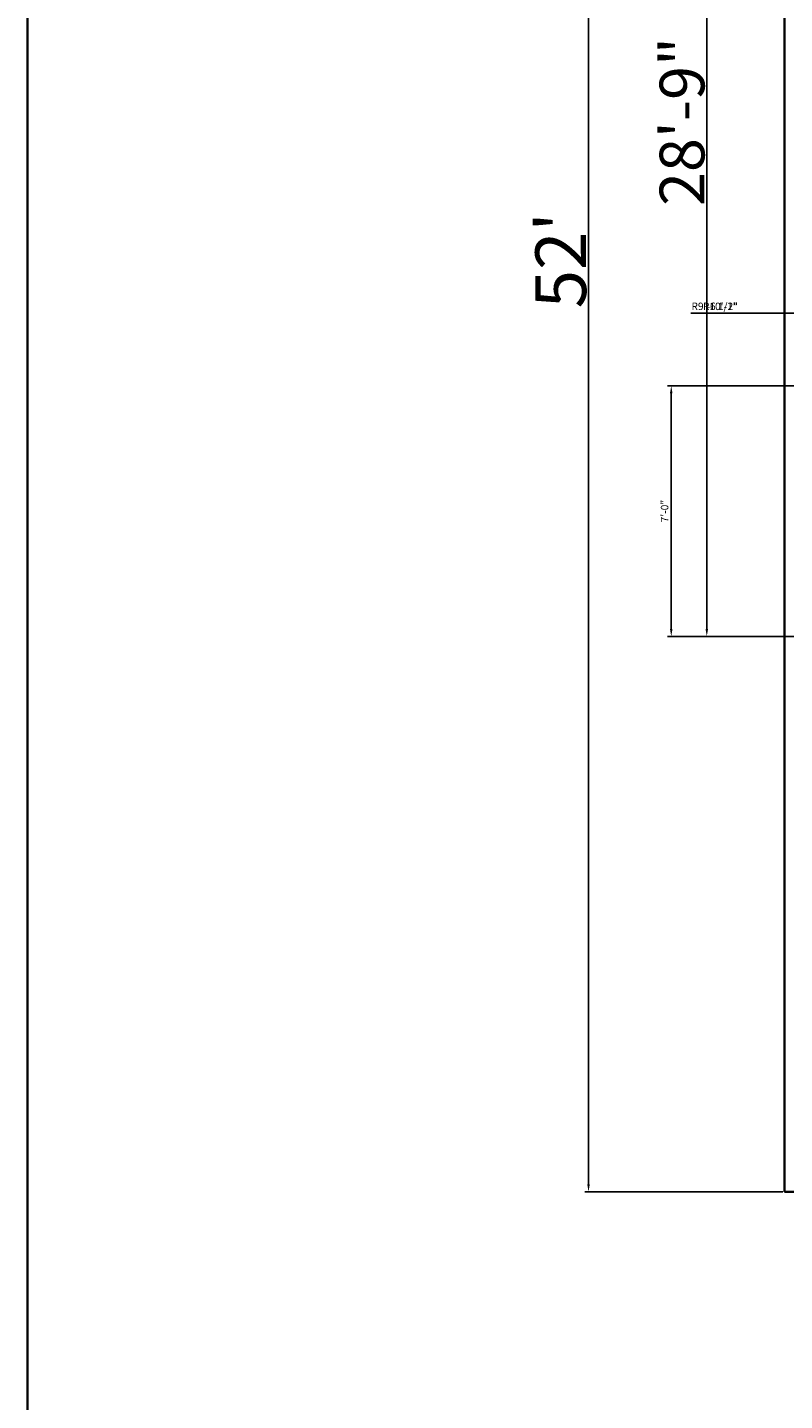
# Model space of a CAD drawing. Units: inches. Extents: x 6038 to 7543, y 3772 to 5131.
# Tile 4 of 14: x 6038 to 6291, y 4293 to 4753. Entities that reach past the tile are written whole.
import ezdxf

# ---------------------------------------------------------------- set-up
doc = ezdxf.new("R2010")
doc.units = ezdxf.units.IN
doc.layers.add('A-ANNO-DIMS', color=4, linetype='Continuous', lineweight=18)
doc.layers.add('A-ANNO-TTLB', color=1, linetype='Continuous', lineweight=35)
doc.layers.add('C-PROP-WALL', color=251, linetype='Continuous', lineweight=35, true_color=0x636466)
doc.styles.get("Standard").update_dxf_attribs({"font": 'arial.ttf'})
doc.dimstyles.new('ISO-25', dxfattribs={"dimtxt": 2.5, "dimasz": 2.5, "dimexe": 1.25, "dimexo": 0.625, "dimtad": 1, "dimdec": 0, "dimlunit": 3, "dimtxsty": 'Standard', "dimcen": 2.5, "dimadec": 0, "dimazin": 0, "dimtfac": 1, "dimtdec": 0, "dimtmove": 0, "dimatfit": 3, "dimfxl": 1, "dimarcsym": 0})

# ---------------------------------------------------------------- blocks, each defined once
blk = doc.blocks.new('*D15')
at = {"layer": 'A-ANNO-DIMS', "color": 0, "lineweight": -2, "transparency": 16777216}
for p, q in [((6320.79, 4893.62), (6264.12, 4893.62)), ((6265.37, 4891.12), (6265.37, 4551.12)), ((6320.79, 4548.62), (6264.12, 4548.62))]:
    blk.add_line(p, q, dxfattribs=at)
at = {"layer": 'A-ANNO-DIMS', "color": 0, "transparency": 16777216}
for points in [[(6264.96, 4891.12), (6265.79, 4891.12), (6265.37, 4893.62)], [(6264.96, 4551.12), (6265.79, 4551.12), (6265.37, 4548.62)]]:
    blk.add_solid(points, dxfattribs=at)
at = {"layer": 'Defpoints', "color": 0, "transparency": 16777216}
for p in [(6321.42, 4893.62), (6265.37, 4548.62), (6321.42, 4548.62)]:
    blk.add_point(p, dxfattribs=at)
at = {"layer": 'A-ANNO-DIMS', "color": 0, "transparency": 16777216, "insert": (6257.09, 4721.12), "char_height": 2.5, "attachment_point": 5, "rotation": 90}
blk.add_mtext('{\\H6x;28\'-9"}', dxfattribs=at)
blk = doc.blocks.new('*D17')
at = {"layer": 'A-ANNO-DIMS', "color": 0, "lineweight": -2, "transparency": 16777216}
for p, q in [((6290.79, 4986.62), (6224.51, 4986.62)), ((6225.76, 4984.12), (6225.76, 4365.12)), ((6290.79, 4362.62), (6224.51, 4362.62))]:
    blk.add_line(p, q, dxfattribs=at)
at = {"layer": 'A-ANNO-DIMS', "color": 0, "transparency": 16777216}
for points in [[(6225.34, 4984.12), (6226.18, 4984.12), (6225.76, 4986.62)], [(6225.34, 4365.12), (6226.18, 4365.12), (6225.76, 4362.62)]]:
    blk.add_solid(points, dxfattribs=at)
at = {"layer": 'Defpoints', "color": 0, "transparency": 16777216}
for p in [(6291.42, 4986.62), (6225.76, 4362.62), (6291.42, 4362.62)]:
    blk.add_point(p, dxfattribs=at)
at = {"layer": 'A-ANNO-DIMS', "color": 0, "transparency": 16777216, "insert": (6216.45, 4674.62), "char_height": 2.5, "attachment_point": 5, "rotation": 90}
blk.add_mtext("{\\H6.8x;52'}", dxfattribs=at)
blk = doc.blocks.new('*D63')
at = {"layer": 'A-ANNO-DIMS', "color": 0, "lineweight": -2, "transparency": 16777216}
for p, q in [((6320.79, 4632.62), (6252.22, 4632.62)), ((6253.47, 4551.12), (6253.47, 4630.12)), ((6320.79, 4548.62), (6252.22, 4548.62))]:
    blk.add_line(p, q, dxfattribs=at)
at = {"layer": 'A-ANNO-DIMS', "color": 0, "transparency": 16777216}
for points in [[(6253.05, 4630.12), (6253.88, 4630.12), (6253.47, 4632.62)], [(6253.05, 4551.12), (6253.88, 4551.12), (6253.47, 4548.62)]]:
    blk.add_solid(points, dxfattribs=at)
at = {"layer": 'Defpoints', "color": 0, "transparency": 16777216}
for p in [(6253.47, 4632.62), (6321.42, 4632.62), (6321.42, 4548.62)]:
    blk.add_point(p, dxfattribs=at)
at = {"layer": 'A-ANNO-DIMS', "color": 0, "transparency": 16777216, "insert": (6251.57, 4590.62), "char_height": 2.5, "attachment_point": 5, "rotation": 90}
blk.add_mtext('7\'-0"', dxfattribs=at)
blk = doc.blocks.new('*D94')
at = {"layer": 'A-ANNO-DIMS', "color": 0, "lineweight": -2, "transparency": 16777216}
for p, q in [((6263.76, 4656.97), (6340.09, 4656.97)), ((6463.79, 4656.97), (6342.59, 4656.97))]:
    blk.add_line(p, q, dxfattribs=at)
at = {"layer": 'A-ANNO-DIMS', "color": 0, "transparency": 16777216}
blk.add_solid([(6340.09, 4657.39), (6340.09, 4656.55), (6342.59, 4656.97)], dxfattribs=at)
at = {"layer": 'Defpoints', "color": 0, "transparency": 16777216}
for p in [(6342.59, 4656.97), (6463.79, 4656.97)]:
    blk.add_point(p, dxfattribs=at)
at = {"layer": 'A-ANNO-DIMS', "color": 0, "transparency": 16777216, "insert": (6269.87, 4658.87), "char_height": 2.5, "attachment_point": 5, "rotation": 0.0002}
blk.add_mtext('R10\'-1"', dxfattribs=at)
blk = doc.blocks.new('*D95')
at = {"layer": 'A-ANNO-DIMS', "color": 0, "lineweight": -2, "transparency": 16777216}
for p, q in [((6259.98, 4656.97), (6334.09, 4656.97)), ((6450.84, 4656.97), (6336.59, 4656.97))]:
    blk.add_line(p, q, dxfattribs=at)
at = {"layer": 'A-ANNO-DIMS', "color": 0, "transparency": 16777216}
blk.add_solid([(6334.09, 4657.39), (6334.09, 4656.55), (6336.59, 4656.97)], dxfattribs=at)
at = {"layer": 'Defpoints', "color": 0, "transparency": 16777216}
for p in [(6336.59, 4656.97), (6450.84, 4656.97)]:
    blk.add_point(p, dxfattribs=at)
at = {"layer": 'A-ANNO-DIMS', "color": 0, "transparency": 16777216, "insert": (6268.04, 4658.89), "char_height": 2.5, "attachment_point": 5, "rotation": 0.0002}
blk.add_mtext('R9\'-6 1/2"', dxfattribs=at)

msp = doc.modelspace()

# ---------------------------------------------------------------- linework, layer by layer
at = {"layer": 'A-ANNO-TTLB'}
msp.add_lwpolyline([(6037.83, 5130.86), (7542.53, 5130.86), (7542.53, 3772.09), (6037.83, 3772.09)], close=True, dxfattribs=at)
at = {"layer": 'C-PROP-WALL'}
for p, q in [((6291.42, 4362.62), (6291.42, 4986.62)), ((6447.42, 4362.62), (6291.42, 4362.62))]:
    msp.add_line(p, q, dxfattribs=at)

# ---------------------------------------------------------------- dimensions: what is measured, and where the dimension line sits
at = {"layer": 'A-ANNO-DIMS'}
dim = msp.add_linear_dim(base=(6225.76, 4362.62), p1=(6291.42, 4986.62), p2=(6291.42, 4362.62), angle=90, text='{\\H6.8x;<>}', dimstyle='ISO-25', override={"dimclrd": 0, "dimclre": 0, "dimclrt": 0}, dxfattribs=at)
dim.commit()
dim.dimension.update_dxf_attribs({"geometry": '*D17', "text_midpoint": (6225.76, 4674.62), "dimtype": 160})
dim = msp.add_linear_dim(base=(6265.37, 4548.62), p1=(6321.42, 4893.62), p2=(6321.42, 4548.62), angle=90, text='{\\H6x;<>}', dimstyle='ISO-25', override={"dimclrd": 0, "dimclre": 0, "dimclrt": 0}, dxfattribs=at)
dim.commit()
dim.dimension.update_dxf_attribs({"geometry": '*D15', "text_midpoint": (6257.09, 4721.12)})
for center, mpoint, picture, middle in [((6450.840765, 4656.970422), (6336.590765, 4656.97), '*D95', (6268.040765, 4656.9697468)), ((6463.79, 4656.97), (6342.59, 4656.97), '*D94', (6269.87, 4656.97))]:
    dim = msp.add_radius_dim(center=center, mpoint=mpoint, dimstyle='ISO-25', override={"dimdec": 1, "dimlfac": 1, "dimrnd": 0, "dimzin": 1, "dimdsep": 46, "dimlunit": 4, "dimfrac": 2}, dxfattribs=at)
    dim.commit()
    dim.dimension.update_dxf_attribs({"geometry": picture, "text_midpoint": middle, "dimtype": 164})
dim = msp.add_linear_dim(base=(6253.47, 4632.62), p1=(6321.42, 4548.62), p2=(6321.42, 4632.62), angle=90, dimstyle='ISO-25', override={"dimdec": 1, "dimlfac": 1, "dimrnd": 0, "dimzin": 1, "dimdsep": 46, "dimlunit": 4, "dimfrac": 2}, dxfattribs=at)
dim.commit()
dim.dimension.update_dxf_attribs({"geometry": '*D63', "text_midpoint": (6251.57, 4590.62)})

doc.saveas('drawing.dxf')
